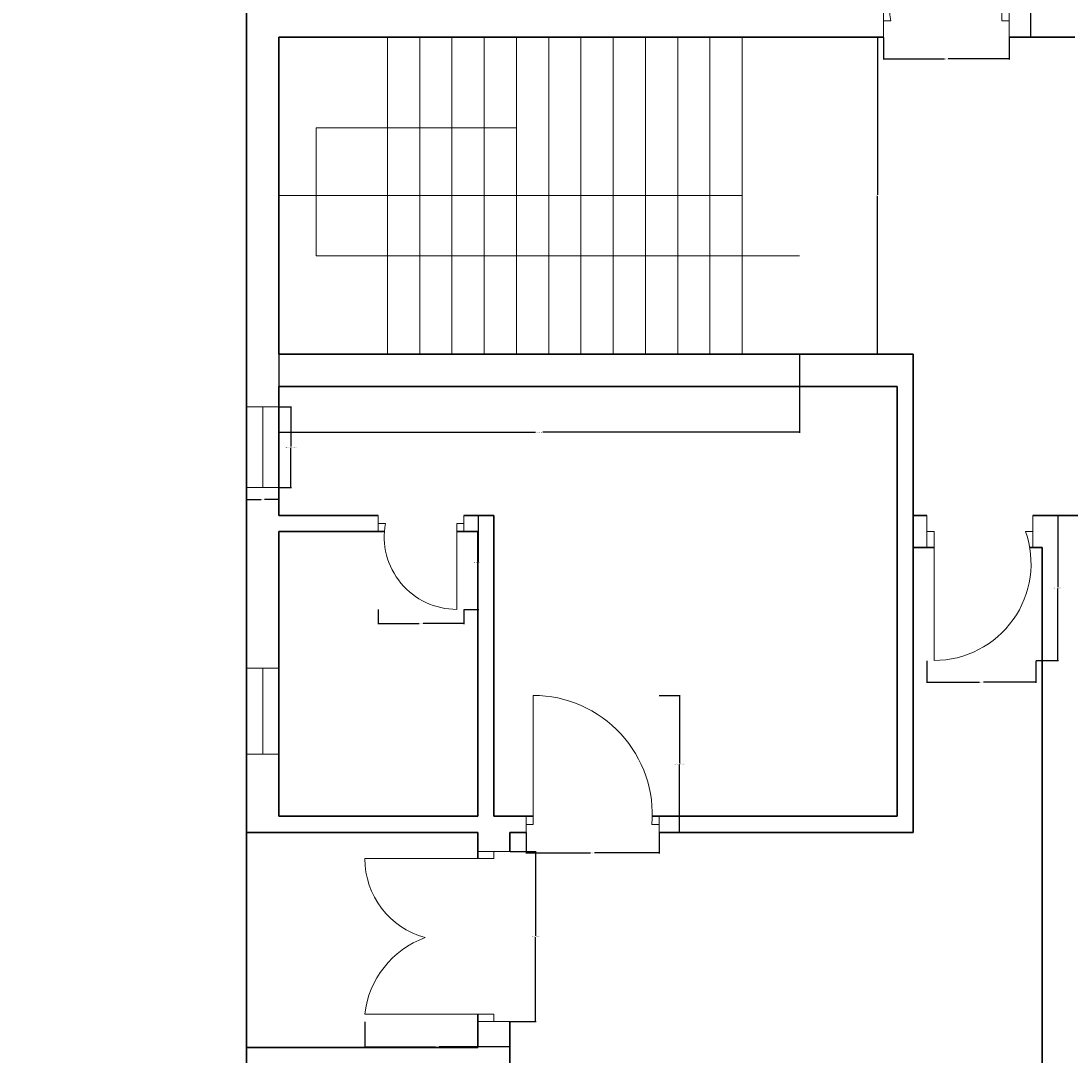
# Model space of a CAD drawing. Units: inches. Extents: x 2250 to 3629, y 982 to 2740.
# Tile 7 of 12: x 2918 to 3211, y 1497 to 1785. Entities that reach past the tile are written whole.
import ezdxf

# ---------------------------------------------------------------- set-up
doc = ezdxf.new("R2010")
doc.units = ezdxf.units.IN
for name, color, linetype, lineweight in [('A-ANNO-DIMS', 2, 'Continuous', 18), ('A-DOOR', 3, 'Continuous', 18), ('A-FLOR-STRS', 7, 'Continuous', 18), ('A-GLAZ', 4, 'Continuous', 18), ('A-WALL', 7, 'Continuous', 35)]:
    doc.layers.add(name, color=color, linetype=linetype, lineweight=lineweight)
doc.styles.get("Standard").update_dxf_attribs({"font": 'arial.ttf'})
doc.dimstyles.get("Standard").update_dxf_attribs({"dimtxt": 0.18, "dimasz": 0.18, "dimexe": 0.18, "dimexo": 0.0625, "dimgap": 0.09, "dimtad": 0, "dimtih": 1, "dimtoh": 1, "dimdec": 4, "dimzin": 0, "dimdsep": 46, "dimtxsty": 'Standard', "dimcen": 0.09, "dimadec": 0, "dimazin": 0, "dimtfac": 1, "dimtdec": 4, "dimtofl": 0, "dimtmove": 0, "dimatfit": 3, "dimfxl": 1, "dimtolj": 1, "dimtzin": 0, "dimarcsym": 0})

# ---------------------------------------------------------------- blocks, each defined once
blk = doc.blocks.new('DR-72-DECK-WEST-S')
for p, q in [((31.5, 47.46), (40.5, 47.46)), ((40.5, 47.46), (36, 47.46)), ((36, 47.46), (36, 45.46)), ((36, 45.46), (0, 45.46)), ((36, 2), (0, 2)), ((36, 0), (36, 2)), ((31.5, 0), (40.5, 0)), ((40.5, 0), (36, 0))]:
    blk.add_line(p, q)
for centre, radius, start, end in [((22.88, 45.46), 22.88, 180, 254.6216), ((25.61, -0.82), 25.77, 109.9642, 173.7115)]:
    blk.add_arc(centre, radius, start, end)
blk = doc.blocks.new('DR-24-BATH-WEST')
for p, q in [((0, 26.25), (0, 21.75)), ((0, 21.75), (0, 24)), ((0, 24), (2, 24)), ((23.91, 24), (21.91, 24)), ((21.91, 24), (21.91, 0)), ((23.91, 21.75), (23.91, 26.25)), ((23.91, 26.25), (23.91, 24))]:
    blk.add_line(p, q)
blk.add_arc((21.91, 20.26), 20.25, 169.3451, 270)
blk = doc.blocks.new('DR-36-BED-WEST')
for p, q in [((2, 2.25), (2, 38.25)), ((0, 4.5), (0, 0)), ((37.11, 4.5), (37.11, 0)), ((0, 0), (0, 2.25)), ((0, 2.25), (2, 2.25)), ((37.11, 2.25), (35.11, 2.25)), ((37.11, 0), (37.11, 2.25))]:
    blk.add_line(p, q)
blk.add_arc((2, 5.02), 33.23, 355.214, 90)
blk = doc.blocks.new('DR-36-ENTRY-SW')
for p, q in [((0, 40.5), (0, 31.5)), ((29.54, 31.5), (29.54, 40.5)), ((0, 31.5), (0, 36)), ((0, 36), (2, 36)), ((2, 36), (2, 0)), ((29.54, 36), (27.54, 36))]:
    blk.add_line(p, q)
blk.add_arc((2, 27.06), 27.06, 270, 19.2844)
blk = doc.blocks.new('DR-36-ENTRY-NW')
for p, q in [((33.05, 4.5), (33.05, 40.5)), ((0, 9.04), (0, 0)), ((35.05, 9.01), (35.05, 0)), ((0, 0), (0, 4.52)), ((0, 4.52), (2, 4.52)), ((35.05, 4.5), (33.05, 4.5)), ((35.05, 0), (35.05, 4.5))]:
    blk.add_line(p, q)
blk.add_arc((33.05, 9.12), 31.39, 90, 188.415)
blk = doc.blocks.new('WIN-24-BATH-NW')
for p, q in [((9, 24), (0, 24)), ((0, 24), (4.5, 24)), ((4.5, 24), (4.5, 0)), ((9, 0), (0, 0)), ((4.5, 0), (9, 0))]:
    blk.add_line(p, q)
blk = doc.blocks.new('WIN-BED-WEST')
for p, q in [((9, 22.49), (0, 22.49)), ((0, 22.49), (4.5, 22.49)), ((4.5, 22.49), (4.5, 0)), ((4.5, 0), (0, 0)), ((0, 0), (9, 0))]:
    blk.add_line(p, q)
blk = doc.blocks.new('STAIR-RETURN-FLIGHT')
for p, q in [((30.31, 88.5), (30.31, 0)), ((39.31, 88.5), (39.31, 0)), ((48.31, 88.5), (48.31, 0)), ((57.31, 88.5), (57.31, 0)), ((66.31, 88.5), (66.31, 0)), ((75.31, 88.5), (75.31, 0)), ((84.31, 88.5), (84.31, 0)), ((93.31, 88.5), (93.31, 0)), ((102.31, 88.5), (102.31, 0)), ((111.31, 88.5), (111.31, 0)), ((120.31, 88.5), (120.31, 0)), ((129.31, 44.25), (129.31, 88.5)), ((129.31, 88.5), (129.31, 0)), ((10.42, 27.46), (10.42, 63.21)), ((10.42, 63.21), (66.31, 63.21)), ((0, 44.25), (129.31, 44.25)), ((145.28, 27.46), (10.42, 27.46))]:
    blk.add_line(p, q)
blk = doc.blocks.new('*D71')
at = {"layer": 'A-ANNO-DIMS', "color": 0, "lineweight": -2, "transparency": 16777216}
for p, q in [((2990.23, 1692.17), (2990.23, 1670.26)), ((3135.5, 1692.17), (3135.5, 1670.26)), ((2990.41, 1670.44), (3061.86, 1670.44)), ((3135.32, 1670.44), (3063.87, 1670.44))]:
    blk.add_line(p, q, dxfattribs=at)
at = {"layer": 'A-ANNO-DIMS', "color": 0, "transparency": 16777216}
for points in [[(2990.41, 1670.47), (2990.41, 1670.41), (2990.23, 1670.44)], [(3135.32, 1670.47), (3135.32, 1670.41), (3135.5, 1670.44)]]:
    blk.add_solid(points, dxfattribs=at)
at = {"layer": 'Defpoints', "color": 0, "transparency": 16777216}
for p in [(2990.23, 1692.24), (3135.5, 1692.24), (3135.5, 1670.44)]:
    blk.add_point(p, dxfattribs=at)
at = {"layer": 'A-ANNO-DIMS', "color": 0, "transparency": 16777216, "insert": (3062.87, 1670.44), "char_height": 0.18, "attachment_point": 5}
blk.add_mtext('\\A1;STAIR 145 TYP.', dxfattribs=at)
blk = doc.blocks.new('*D72')
at = {"layer": 'A-ANNO-DIMS', "color": 0, "lineweight": -2, "transparency": 16777216}
for p, q in [((3135.57, 1780.74), (3157.48, 1780.74)), ((3157.3, 1780.56), (3157.3, 1736.67)), ((3157.3, 1692.42), (3157.3, 1736.3)), ((3135.57, 1692.24), (3157.48, 1692.24))]:
    blk.add_line(p, q, dxfattribs=at)
at = {"layer": 'A-ANNO-DIMS', "color": 0, "transparency": 16777216}
for points in [[(3157.27, 1780.56), (3157.33, 1780.56), (3157.3, 1780.74)], [(3157.27, 1692.42), (3157.33, 1692.42), (3157.3, 1692.24)]]:
    blk.add_solid(points, dxfattribs=at)
at = {"layer": 'Defpoints', "color": 0, "transparency": 16777216}
for p in [(3135.5, 1780.74), (3157.3, 1780.74), (3135.5, 1692.24)]:
    blk.add_point(p, dxfattribs=at)
at = {"layer": 'A-ANNO-DIMS', "color": 0, "transparency": 16777216, "insert": (3157.3, 1736.49), "char_height": 0.18, "attachment_point": 5}
blk.add_mtext('\\A1;89 TYP.', dxfattribs=at)
blk = doc.blocks.new('*D95')
at = {"layer": 'A-ANNO-DIMS', "color": 0, "lineweight": -2, "transparency": 16777216}
for p, q in [((2990.29, 1677.5), (2993.78, 1677.5)), ((2993.6, 1677.32), (2993.6, 1666.44)), ((2993.6, 1655.2), (2993.6, 1666.08)), ((2990.29, 1655.02), (2993.78, 1655.02))]:
    blk.add_line(p, q, dxfattribs=at)
at = {"layer": 'A-ANNO-DIMS', "color": 0, "transparency": 16777216}
for points in [[(2993.57, 1677.32), (2993.63, 1677.32), (2993.6, 1677.5)], [(2993.57, 1655.2), (2993.63, 1655.2), (2993.6, 1655.02)]]:
    blk.add_solid(points, dxfattribs=at)
at = {"layer": 'Defpoints', "color": 0, "transparency": 16777216}
for p in [(2990.23, 1677.5), (2993.6, 1677.5), (2990.23, 1655.02)]:
    blk.add_point(p, dxfattribs=at)
at = {"layer": 'A-ANNO-DIMS', "color": 0, "transparency": 16777216, "insert": (2993.6, 1666.26), "char_height": 0.18, "attachment_point": 5}
blk.add_mtext('\\A1;BEDROOM WINDOW 22 TYP.', dxfattribs=at)
blk = doc.blocks.new('*D96')
at = {"layer": 'A-ANNO-DIMS', "color": 0, "lineweight": -2, "transparency": 16777216}
for p, q in [((2981.23, 1654.95), (2981.23, 1651.46)), ((2990.23, 1654.95), (2990.23, 1651.46)), ((2981.41, 1651.64), (2985.27, 1651.64)), ((2990.05, 1651.64), (2986.18, 1651.64))]:
    blk.add_line(p, q, dxfattribs=at)
at = {"layer": 'A-ANNO-DIMS', "color": 0, "transparency": 16777216}
for points in [[(2981.41, 1651.67), (2981.41, 1651.61), (2981.23, 1651.64)], [(2990.05, 1651.67), (2990.05, 1651.61), (2990.23, 1651.64)]]:
    blk.add_solid(points, dxfattribs=at)
at = {"layer": 'Defpoints', "color": 0, "transparency": 16777216}
for p in [(2981.23, 1655.02), (2990.23, 1655.02), (2990.23, 1651.64)]:
    blk.add_point(p, dxfattribs=at)
at = {"layer": 'A-ANNO-DIMS', "color": 0, "transparency": 16777216, "insert": (2985.73, 1651.64), "char_height": 0.18, "attachment_point": 5}
blk.add_mtext('\\A1;9 TYP.', dxfattribs=at)
blk = doc.blocks.new('*D125')
at = {"layer": 'A-ANNO-DIMS', "color": 0, "lineweight": -2, "transparency": 16777216}
for p, q in [((3054.79, 1553.42), (3062.03, 1553.42)), ((3061.85, 1553.24), (3061.85, 1529.88)), ((3061.85, 1506.14), (3061.85, 1529.51)), ((3054.79, 1505.96), (3062.03, 1505.96))]:
    blk.add_line(p, q, dxfattribs=at)
at = {"layer": 'A-ANNO-DIMS', "color": 0, "transparency": 16777216}
for points in [[(3061.82, 1553.24), (3061.88, 1553.24), (3061.85, 1553.42)], [(3061.82, 1506.14), (3061.88, 1506.14), (3061.85, 1505.96)]]:
    blk.add_solid(points, dxfattribs=at)
at = {"layer": 'Defpoints', "color": 0, "transparency": 16777216}
for p in [(3054.73, 1553.42), (3061.85, 1553.42), (3054.73, 1505.96)]:
    blk.add_point(p, dxfattribs=at)
at = {"layer": 'A-ANNO-DIMS', "color": 0, "transparency": 16777216, "insert": (3061.85, 1529.69), "char_height": 0.18, "attachment_point": 5}
blk.add_mtext('\\A1;DECK DOOR 47 TYP.', dxfattribs=at)
blk = doc.blocks.new('*D126')
at = {"layer": 'A-ANNO-DIMS', "color": 0, "lineweight": -2, "transparency": 16777216}
for p, q in [((3014.23, 1505.9), (3014.23, 1498.67)), ((3054.73, 1505.9), (3054.73, 1498.67)), ((3014.41, 1498.85), (3033.95, 1498.85)), ((3054.55, 1498.85), (3035.01, 1498.85))]:
    blk.add_line(p, q, dxfattribs=at)
at = {"layer": 'A-ANNO-DIMS', "color": 0, "transparency": 16777216}
for points in [[(3014.41, 1498.88), (3014.41, 1498.82), (3014.23, 1498.85)], [(3054.55, 1498.88), (3054.55, 1498.82), (3054.73, 1498.85)]]:
    blk.add_solid(points, dxfattribs=at)
at = {"layer": 'Defpoints', "color": 0, "transparency": 16777216}
for p in [(3014.23, 1505.96), (3054.73, 1505.96), (3054.73, 1498.85)]:
    blk.add_point(p, dxfattribs=at)
at = {"layer": 'A-ANNO-DIMS', "color": 0, "transparency": 16777216, "insert": (3034.48, 1498.85), "char_height": 0.18, "attachment_point": 5}
blk.add_mtext('\\A1;41 TYP.', dxfattribs=at)
blk = doc.blocks.new('*D127')
at = {"layer": 'A-ANNO-DIMS', "color": 0, "lineweight": -2, "transparency": 16777216}
for p, q in [((3041.94, 1647.24), (3046, 1647.24)), ((3045.82, 1647.06), (3045.82, 1634.29)), ((3045.82, 1621.17), (3045.82, 1633.93)), ((3041.94, 1620.99), (3046, 1620.99))]:
    blk.add_line(p, q, dxfattribs=at)
at = {"layer": 'A-ANNO-DIMS', "color": 0, "transparency": 16777216}
for points in [[(3045.79, 1647.06), (3045.85, 1647.06), (3045.82, 1647.24)], [(3045.79, 1621.17), (3045.85, 1621.17), (3045.82, 1620.99)]]:
    blk.add_solid(points, dxfattribs=at)
at = {"layer": 'Defpoints', "color": 0, "transparency": 16777216}
for p in [(3041.88, 1647.24), (3045.82, 1647.24), (3041.88, 1620.99)]:
    blk.add_point(p, dxfattribs=at)
at = {"layer": 'A-ANNO-DIMS', "color": 0, "transparency": 16777216, "insert": (3045.82, 1634.11), "char_height": 0.18, "attachment_point": 5}
blk.add_mtext('\\A1;BATH DOOR 26 TYP.', dxfattribs=at)
blk = doc.blocks.new('*D128')
at = {"layer": 'A-ANNO-DIMS', "color": 0, "lineweight": -2, "transparency": 16777216}
for p, q in [((3017.98, 1620.92), (3017.98, 1616.87)), ((3041.88, 1620.92), (3041.88, 1616.87)), ((3018.16, 1617.05), (3029.4, 1617.05)), ((3041.7, 1617.05), (3030.46, 1617.05))]:
    blk.add_line(p, q, dxfattribs=at)
at = {"layer": 'A-ANNO-DIMS', "color": 0, "transparency": 16777216}
for points in [[(3018.16, 1617.08), (3018.16, 1617.02), (3017.98, 1617.05)], [(3041.7, 1617.08), (3041.7, 1617.02), (3041.88, 1617.05)]]:
    blk.add_solid(points, dxfattribs=at)
at = {"layer": 'Defpoints', "color": 0, "transparency": 16777216}
for p in [(3017.98, 1620.99), (3041.88, 1620.99), (3041.88, 1617.05)]:
    blk.add_point(p, dxfattribs=at)
at = {"layer": 'A-ANNO-DIMS', "color": 0, "transparency": 16777216, "insert": (3029.93, 1617.05), "char_height": 0.18, "attachment_point": 5}
blk.add_mtext('\\A1;24 TYP.', dxfattribs=at)
blk = doc.blocks.new('*D129')
at = {"layer": 'A-ANNO-DIMS', "color": 0, "lineweight": -2, "transparency": 16777216}
for p, q in [((3096.38, 1596.99), (3102.24, 1596.99)), ((3102.06, 1596.81), (3102.06, 1578.04)), ((3102.06, 1558.92), (3102.06, 1577.68)), ((3096.38, 1558.74), (3102.24, 1558.74))]:
    blk.add_line(p, q, dxfattribs=at)
at = {"layer": 'A-ANNO-DIMS', "color": 0, "transparency": 16777216}
for points in [[(3102.03, 1596.81), (3102.09, 1596.81), (3102.06, 1596.99)], [(3102.03, 1558.92), (3102.09, 1558.92), (3102.06, 1558.74)]]:
    blk.add_solid(points, dxfattribs=at)
at = {"layer": 'Defpoints', "color": 0, "transparency": 16777216}
for p in [(3096.32, 1596.99), (3102.06, 1596.99), (3096.32, 1558.74)]:
    blk.add_point(p, dxfattribs=at)
at = {"layer": 'A-ANNO-DIMS', "color": 0, "transparency": 16777216, "insert": (3102.06, 1577.86), "char_height": 0.18, "attachment_point": 5}
blk.add_mtext('\\A1;BEDROOM DOOR 38 TYP.', dxfattribs=at)
blk = doc.blocks.new('*D130')
at = {"layer": 'A-ANNO-DIMS', "color": 0, "lineweight": -2, "transparency": 16777216}
for p, q in [((3059.21, 1558.67), (3059.21, 1552.82)), ((3096.32, 1558.67), (3096.32, 1552.82)), ((3059.39, 1553), (3077.23, 1553)), ((3096.14, 1553), (3078.29, 1553))]:
    blk.add_line(p, q, dxfattribs=at)
at = {"layer": 'A-ANNO-DIMS', "color": 0, "transparency": 16777216}
for points in [[(3059.39, 1553.03), (3059.39, 1552.97), (3059.21, 1553)], [(3096.14, 1553.03), (3096.14, 1552.97), (3096.32, 1553)]]:
    blk.add_solid(points, dxfattribs=at)
at = {"layer": 'Defpoints', "color": 0, "transparency": 16777216}
for p in [(3059.21, 1558.74), (3096.32, 1558.74), (3096.32, 1553)]:
    blk.add_point(p, dxfattribs=at)
at = {"layer": 'A-ANNO-DIMS', "color": 0, "transparency": 16777216, "insert": (3077.76, 1553), "char_height": 0.18, "attachment_point": 5}
blk.add_mtext('\\A1;37 TYP.', dxfattribs=at)
blk = doc.blocks.new('*D135')
at = {"layer": 'A-ANNO-DIMS', "color": 0, "lineweight": -2, "transparency": 16777216}
for p, q in [((3201.57, 1647.24), (3207.77, 1647.24)), ((3207.59, 1647.06), (3207.59, 1627.17)), ((3207.59, 1606.92), (3207.59, 1626.8)), ((3201.57, 1606.74), (3207.77, 1606.74))]:
    blk.add_line(p, q, dxfattribs=at)
at = {"layer": 'A-ANNO-DIMS', "color": 0, "transparency": 16777216}
for points in [[(3207.56, 1647.06), (3207.62, 1647.06), (3207.59, 1647.24)], [(3207.56, 1606.92), (3207.62, 1606.92), (3207.59, 1606.74)]]:
    blk.add_solid(points, dxfattribs=at)
at = {"layer": 'Defpoints', "color": 0, "transparency": 16777216}
for p in [(3201.51, 1647.24), (3207.59, 1647.24), (3201.51, 1606.74)]:
    blk.add_point(p, dxfattribs=at)
at = {"layer": 'A-ANNO-DIMS', "color": 0, "transparency": 16777216, "insert": (3207.59, 1626.99), "char_height": 0.18, "attachment_point": 5}
blk.add_mtext('\\A1;ENTRY DOOR 41 TYP.', dxfattribs=at)
blk = doc.blocks.new('*D136')
at = {"layer": 'A-ANNO-DIMS', "color": 0, "lineweight": -2, "transparency": 16777216}
for p, q in [((3171.07, 1606.67), (3171.07, 1600.48)), ((3201.51, 1606.67), (3201.51, 1600.48)), ((3171.25, 1600.66), (3185.76, 1600.66)), ((3201.33, 1600.66), (3186.82, 1600.66))]:
    blk.add_line(p, q, dxfattribs=at)
at = {"layer": 'A-ANNO-DIMS', "color": 0, "transparency": 16777216}
for points in [[(3171.25, 1600.69), (3171.25, 1600.63), (3171.07, 1600.66)], [(3201.33, 1600.69), (3201.33, 1600.63), (3201.51, 1600.66)]]:
    blk.add_solid(points, dxfattribs=at)
at = {"layer": 'Defpoints', "color": 0, "transparency": 16777216}
for p in [(3171.07, 1606.74), (3201.51, 1606.74), (3201.51, 1600.66)]:
    blk.add_point(p, dxfattribs=at)
at = {"layer": 'A-ANNO-DIMS', "color": 0, "transparency": 16777216, "insert": (3186.29, 1600.66), "char_height": 0.18, "attachment_point": 5}
blk.add_mtext('\\A1;30 TYP.', dxfattribs=at)
blk = doc.blocks.new('*D137')
at = {"layer": 'A-ANNO-DIMS', "color": 0, "lineweight": -2, "transparency": 16777216}
for p, q in [((3194.07, 1821.24), (3200.27, 1821.24)), ((3200.09, 1821.06), (3200.09, 1801.17)), ((3200.09, 1780.92), (3200.09, 1800.8)), ((3194.07, 1780.74), (3200.27, 1780.74))]:
    blk.add_line(p, q, dxfattribs=at)
at = {"layer": 'A-ANNO-DIMS', "color": 0, "transparency": 16777216}
for points in [[(3200.06, 1821.06), (3200.12, 1821.06), (3200.09, 1821.24)], [(3200.06, 1780.92), (3200.12, 1780.92), (3200.09, 1780.74)]]:
    blk.add_solid(points, dxfattribs=at)
at = {"layer": 'Defpoints', "color": 0, "transparency": 16777216}
for p in [(3194.01, 1821.24), (3200.09, 1821.24), (3194.01, 1780.74)]:
    blk.add_point(p, dxfattribs=at)
at = {"layer": 'A-ANNO-DIMS', "color": 0, "transparency": 16777216, "insert": (3200.09, 1800.99), "char_height": 0.18, "attachment_point": 5}
blk.add_mtext('\\A1;ENTRY DOOR 41 TYP.', dxfattribs=at)
blk = doc.blocks.new('*D138')
at = {"layer": 'A-ANNO-DIMS', "color": 0, "lineweight": -2, "transparency": 16777216}
for p, q in [((3158.96, 1780.67), (3158.96, 1774.48)), ((3194.01, 1780.67), (3194.01, 1774.48)), ((3159.14, 1774.66), (3175.96, 1774.66)), ((3193.83, 1774.66), (3177.01, 1774.66))]:
    blk.add_line(p, q, dxfattribs=at)
at = {"layer": 'A-ANNO-DIMS', "color": 0, "transparency": 16777216}
for points in [[(3159.14, 1774.69), (3159.14, 1774.63), (3158.96, 1774.66)], [(3193.83, 1774.69), (3193.83, 1774.63), (3194.01, 1774.66)]]:
    blk.add_solid(points, dxfattribs=at)
at = {"layer": 'Defpoints', "color": 0, "transparency": 16777216}
for p in [(3158.96, 1780.74), (3194.01, 1780.74), (3194.01, 1774.66)]:
    blk.add_point(p, dxfattribs=at)
at = {"layer": 'A-ANNO-DIMS', "color": 0, "transparency": 16777216, "insert": (3176.49, 1774.66), "char_height": 0.18, "attachment_point": 5}
blk.add_mtext('\\A1;35 TYP.', dxfattribs=at)
blk = doc.blocks.new('*D172')
at = {"layer": 'A-ANNO-DIMS', "color": 0, "lineweight": -2, "transparency": 16777216}
for p, q in [((3433.02, 2070.24), (3541.21, 2070.24)), ((3541.03, 2070.06), (3541.03, 1664.67)), ((3541.03, 1258.92), (3541.03, 1664.3)), ((3059.29, 1258.74), (3541.21, 1258.74))]:
    blk.add_line(p, q, dxfattribs=at)
at = {"layer": 'A-ANNO-DIMS', "color": 0, "transparency": 16777216}
for points in [[(3541, 2070.06), (3541.06, 2070.06), (3541.03, 2070.24)], [(3541, 1258.92), (3541.06, 1258.92), (3541.03, 1258.74)]]:
    blk.add_solid(points, dxfattribs=at)
at = {"layer": 'Defpoints', "color": 0, "transparency": 16777216}
for p in [(3432.96, 2070.24), (3541.03, 2070.24), (3059.23, 1258.74)]:
    blk.add_point(p, dxfattribs=at)
at = {"layer": 'A-ANNO-DIMS', "color": 0, "transparency": 16777216, "insert": (3541.03, 1664.49), "char_height": 0.18, "attachment_point": 5}
blk.add_mtext('\\A1;811.5', dxfattribs=at)
blk = doc.blocks.new('*D173')
at = {"layer": 'A-ANNO-DIMS', "color": 0, "lineweight": -2, "transparency": 16777216}
for p, q in [((2932.01, 1947.92), (2890.14, 1947.92)), ((2890.32, 1947.74), (2890.32, 1603.51)), ((2890.32, 1258.92), (2890.32, 1603.15)), ((2981.16, 1258.74), (2890.14, 1258.74))]:
    blk.add_line(p, q, dxfattribs=at)
at = {"layer": 'A-ANNO-DIMS', "color": 0, "transparency": 16777216}
for points in [[(2890.29, 1947.74), (2890.35, 1947.74), (2890.32, 1947.92)], [(2890.29, 1258.92), (2890.35, 1258.92), (2890.32, 1258.74)]]:
    blk.add_solid(points, dxfattribs=at)
at = {"layer": 'Defpoints', "color": 0, "transparency": 16777216}
for p in [(2932.07, 1947.92), (2890.32, 1258.74), (2981.23, 1258.74)]:
    blk.add_point(p, dxfattribs=at)
at = {"layer": 'A-ANNO-DIMS', "color": 0, "transparency": 16777216, "insert": (2890.32, 1603.33), "char_height": 0.18, "attachment_point": 5}
blk.add_mtext('\\A1;689.2', dxfattribs=at)

msp = doc.modelspace()

# ---------------------------------------------------------------- linework, layer by layer
at = {"layer": 'A-WALL'}
for p, q in [((2981.2267, 2047.7354), (2981.2267, 1276.7354)), ((2990.2267, 1780.7354), (2990.2267, 1692.2354)), ((2990.2267, 1780.7354), (3054.7267, 1780.7354)), ((3054.7267, 1780.7354), (3158.9612, 1780.7354)), ((3194.0123, 1780.7354), (3203.2267, 1780.7354)), ((3212.321, 1780.7354), (3203.2267, 1780.7354)), ((2990.2267, 1692.2354), (3162.7267, 1692.2354)), ((3162.7267, 1692.2354), (3167.2267, 1692.2354)), ((3167.2267, 1692.2354), (3167.2267, 1563.2354)), ((2990.2267, 1683.2354), (2990.2267, 1647.2354)), ((3162.7267, 1683.2354), (2990.2267, 1683.2354)), ((3162.7267, 1563.2354), (3162.7267, 1683.2354)), ((2990.2267, 1647.2354), (3017.9767, 1647.2354)), ((3041.8825, 1647.2354), (3045.7267, 1647.2354)), ((3045.7267, 1647.2354), (3050.2267, 1647.2354)), ((3050.2267, 1647.2354), (3050.2267, 1618.7354)), ((3171.0712, 1647.2354), (3167.2267, 1647.2354)), ((3167.2267, 1647.2354), (3167.2267, 1638.2354)), ((3224.6679, 1647.2354), (3200.6151, 1647.2354)), ((2990.2267, 1642.7354), (2990.2267, 1563.2354)), ((3019.6828, 1642.7354), (2990.2267, 1642.7354)), ((3045.7267, 1642.7354), (3039.8825, 1642.7354)), ((3045.7267, 1563.2354), (3045.7267, 1642.7354)), ((3167.2267, 1638.2354), (3173.0712, 1638.2354)), ((3199.7673, 1638.2354), (3203.2267, 1638.2354)), ((3203.2267, 1638.2354), (3203.2267, 1434.2354)), ((3050.2267, 1563.2354), (3050.2267, 1618.7354)), ((2990.2267, 1563.2354), (3045.7267, 1563.2354)), ((3050.2267, 1563.2354), (3054.7267, 1563.2354)), ((3054.7267, 1563.2354), (3061.2061, 1563.2354)), ((3094.4297, 1563.2354), (3162.7267, 1563.2354)), ((3167.2267, 1563.2354), (3167.2267, 1558.7354)), ((2990.2267, 1558.7354), (2981.2267, 1558.7354)), ((2990.2267, 1558.7354), (3045.7267, 1558.7354)), ((3045.7267, 1558.7354), (3045.7267, 1551.4204)), ((3054.7267, 1553.4204), (3054.7267, 1558.7354)), ((3059.2061, 1558.7354), (3054.7267, 1558.7354)), ((3167.2267, 1558.7354), (3096.318, 1558.7354)), ((3045.7267, 1507.9638), (3045.7267, 1498.7354)), ((3054.7267, 1498.7354), (3054.7267, 1505.9638)), ((2990.2267, 1498.7354), (2981.2267, 1498.7354)), ((2990.2267, 1498.7354), (3045.7267, 1498.7354)), ((3054.7267, 1498.7354), (3054.7267, 1487.263))]:
    msp.add_line(p, q, dxfattribs=at)

# ---------------------------------------------------------------- block references
at = {"layer": 'A-DOOR'}
for name, p in [('DR-36-ENTRY-NW', (3158.9615, 1780.735)), ('DR-24-BATH-WEST', (3017.9765, 1620.985)), ('DR-36-ENTRY-SW', (3171.0715, 1606.735)), ('DR-36-BED-WEST', (3059.2065, 1558.735)), ('DR-72-DECK-WEST-S', (3014.2265, 1505.964))]:
    msp.add_blockref(name, p, dxfattribs=at)
at = {"layer": 'A-FLOR-STRS'}
msp.add_blockref('STAIR-RETURN-FLIGHT', (2990.2265, 1692.235), dxfattribs=at)
at = {"layer": 'A-GLAZ'}
msp.add_blockref('WIN-BED-WEST', (2981.2265, 1655.016), dxfattribs=at)
at = {"layer": 'A-GLAZ', "rotation": 180}
msp.add_blockref('WIN-24-BATH-NW', (2990.2269, 1604.5739), dxfattribs=at)

# ---------------------------------------------------------------- dimensions: what is measured, and where the dimension line sits
at = {"layer": 'A-ANNO-DIMS'}
for base, p1, p2, picture, middle in [((3541.0278, 2070.2354), (3059.2267, 1258.7354), (3432.9579, 2070.2354), '*D172', (3541.0278, 1664.4854)), ((2890.3241, 1258.7354), (2932.0741, 1947.9231), (2981.2267, 1258.7354), '*D173', (2890.3241, 1603.3293))]:
    dim = msp.add_linear_dim(base=base, p1=p1, p2=p2, angle=90, dimstyle='Standard', override={"dimdec": 1, "dimlfac": 1, "dimrnd": 0, "dimzin": 0, "dimdsep": 46, "dimlunit": 2}, dxfattribs=at)
    dim.commit()
    dim.dimension.update_dxf_attribs({"geometry": picture, "text_midpoint": middle})
for base, p1, p2, text, picture, middle in [((3200.088, 1821.24), (3194.0123, 1780.7354), (3194.0123, 1821.24), 'ENTRY DOOR <> TYP.', '*D137', (3200.088, 1800.9877)), ((3157.2950108184, 1780.7354249075), (3135.503495462, 1692.2354249075), (3135.503495462, 1780.7354249075), '<> TYP.', '*D72', (3157.2950108184, 1736.4854249075)), ((2993.5998, 1677.5031), (2990.2267, 1655.0159), (2990.2267, 1677.5031), 'BEDROOM WINDOW <> TYP.', '*D95', (2993.5998, 1666.2595)), ((3045.82, 1647.2354), (3041.8825, 1620.9854), (3041.8825, 1647.2354), 'BATH DOOR <> TYP.', '*D127', (3045.82, 1634.1104)), ((3207.5864341643, 1647.2354249075), (3201.5114341643, 1606.7354249075), (3201.5114341643, 1647.2354249075), 'ENTRY DOOR <> TYP.', '*D135', (3207.5864341643, 1626.9854249075)), ((3102.0555, 1596.9854), (3096.318, 1558.7354), (3096.318, 1596.9854), 'BEDROOM DOOR <> TYP.', '*D129', (3102.0555, 1577.8604)), ((3061.8452, 1553.4204), (3054.7267, 1505.9638), (3054.7267, 1553.4204), 'DECK DOOR <> TYP.', '*D125', (3061.8452, 1529.6921))]:
    dim = msp.add_linear_dim(base=base, p1=p1, p2=p2, angle=90, text=text, dimstyle='Standard', override={"dimdec": 0, "dimlfac": 1, "dimrnd": 0, "dimzin": 0, "dimdsep": 46, "dimlunit": 2}, dxfattribs=at)
    dim.commit()
    dim.dimension.update_dxf_attribs({"geometry": picture, "text_midpoint": middle})
for base, p1, p2, text, picture, middle in [((3194.0123, 1774.6597), (3158.9612, 1780.7354), (3194.0123, 1780.7354), '<> TYP.', '*D138', (3176.4867, 1774.6597)), ((3135.5035, 1670.4439), (2990.2267, 1692.2354), (3135.5035, 1692.2354), 'STAIR <> TYP.', '*D71', (3062.8651, 1670.4439)), ((2990.2267, 1651.6428), (2981.2267, 1655.0159), (2990.2267, 1655.0159), '<> TYP.', '*D96', (2985.7267, 1651.6428)), ((3041.8825, 1617.0479), (3017.9767, 1620.9854), (3041.8825, 1620.9854), '<> TYP.', '*D128', (3029.9296, 1617.0479)), ((3201.5114, 1600.6604), (3171.0712, 1606.7354), (3201.5114, 1606.7354), '<> TYP.', '*D136', (3186.2913, 1600.6604)), ((3096.318, 1552.9979), (3059.2061, 1558.7354), (3096.318, 1558.7354), '<> TYP.', '*D130', (3077.762, 1552.9979)), ((3054.726726419, 1498.8453284208), (3014.226726419, 1505.9638212118), (3054.726726419, 1505.9638212118), '<> TYP.', '*D126', (3034.476726419, 1498.8453284208))]:
    dim = msp.add_linear_dim(base=base, p1=p1, p2=p2, text=text, dimstyle='Standard', override={"dimdec": 0, "dimlfac": 1, "dimrnd": 0, "dimzin": 0, "dimdsep": 46, "dimlunit": 2}, dxfattribs=at)
    dim.commit()
    dim.dimension.update_dxf_attribs({"geometry": picture, "text_midpoint": middle})

doc.saveas('drawing.dxf')
